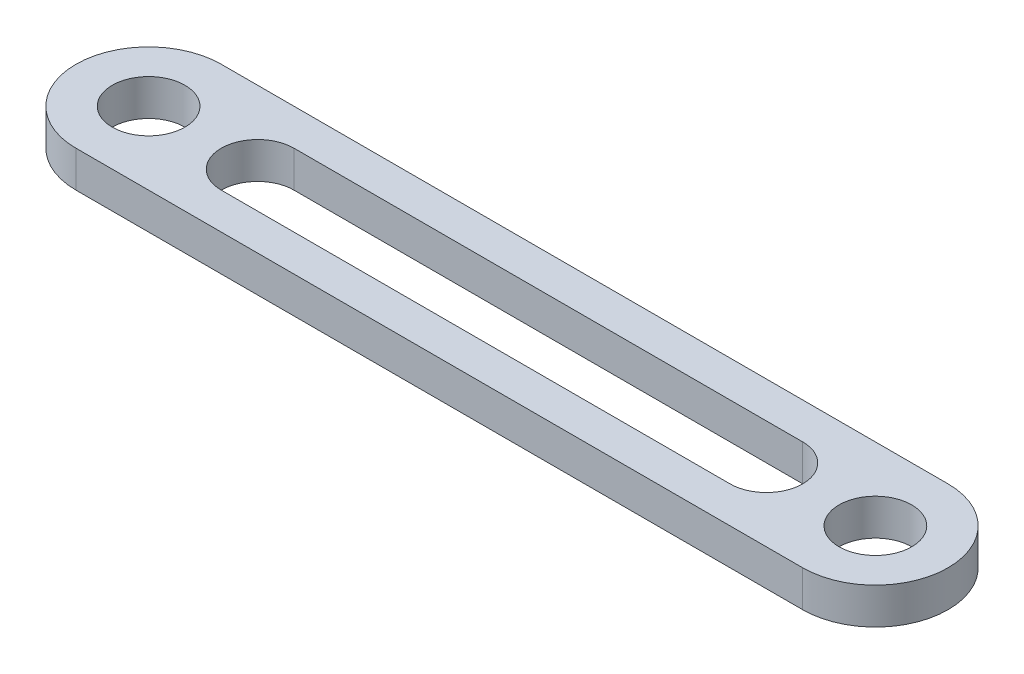
ISO-10303-21;
HEADER;
FILE_DESCRIPTION(('STEP AP214'),'2;1');
FILE_NAME('part.step','',(''),(''),'','','');
FILE_SCHEMA(('AUTOMOTIVE_DESIGN { 1 0 10303 214 1 1 1 1 }'));
ENDSEC;
DATA;
#1=APPLICATION_CONTEXT('core data for automotive mechanical design processes');
#2=APPLICATION_PROTOCOL_DEFINITION('international standard','automotive_design',2000,#1);
#3=PRODUCT_CONTEXT('',#1,'mechanical');
#4=PRODUCT('Part','Part','',(#3));
#5=PRODUCT_RELATED_PRODUCT_CATEGORY('part','',(#4));
#6=PRODUCT_DEFINITION_FORMATION('','',#4);
#7=PRODUCT_DEFINITION_CONTEXT('part definition',#1,'design');
#8=PRODUCT_DEFINITION('design','',#6,#7);
#9=PRODUCT_DEFINITION_SHAPE('','',#8);
#10=(LENGTH_UNIT() NAMED_UNIT(*) SI_UNIT(.MILLI.,.METRE.));
#11=(NAMED_UNIT(*) PLANE_ANGLE_UNIT() SI_UNIT($,.RADIAN.));
#12=(NAMED_UNIT(*) SI_UNIT($,.STERADIAN.) SOLID_ANGLE_UNIT());
#13=UNCERTAINTY_MEASURE_WITH_UNIT(LENGTH_MEASURE(1.E-05),#10,'distance_accuracy_value','');
#14=(GEOMETRIC_REPRESENTATION_CONTEXT(3) GLOBAL_UNCERTAINTY_ASSIGNED_CONTEXT((#13)) GLOBAL_UNIT_ASSIGNED_CONTEXT((#10,
#11,#12)) REPRESENTATION_CONTEXT('',''));
#15=CARTESIAN_POINT('',(0.,0.,0.));
#16=DIRECTION('',(0.,0.,1.));
#17=DIRECTION('',(1.,0.,0.));
#18=AXIS2_PLACEMENT_3D('',#15,#16,#17);
#19=CARTESIAN_POINT('',(-50.,5.,0.));
#20=DIRECTION('',(0.,1.,0.));
#21=DIRECTION('',(0.,0.,1.));
#22=AXIS2_PLACEMENT_3D('',#19,#20,#21);
#23=PLANE('',#22);
#24=CARTESIAN_POINT('',(-50.,5.,0.));
#25=DIRECTION('',(0.,1.,0.));
#26=DIRECTION('',(0.,0.,1.));
#27=AXIS2_PLACEMENT_3D('',#24,#25,#26);
#28=CIRCLE('',#27,5.);
#29=CARTESIAN_POINT('',(-50.,5.,5.));
#30=VERTEX_POINT('',#29);
#31=EDGE_CURVE('E148',#30,#30,#28,.T.);
#32=ORIENTED_EDGE('',*,*,#31,.F.);
#33=EDGE_LOOP('',(#32));
#34=FACE_BOUND('',#33,.T.);
#35=CARTESIAN_POINT('',(-50.,5.,0.));
#36=DIRECTION('',(0.,1.,0.));
#37=DIRECTION('',(0.,0.,1.));
#38=AXIS2_PLACEMENT_3D('',#35,#36,#37);
#39=CIRCLE('',#38,10.);
#40=CARTESIAN_POINT('',(-50.,5.,-10.));
#41=VERTEX_POINT('',#40);
#42=CARTESIAN_POINT('',(-50.,5.,10.));
#43=VERTEX_POINT('',#42);
#44=EDGE_CURVE('E155',#41,#43,#39,.T.);
#45=ORIENTED_EDGE('',*,*,#44,.T.);
#46=DIRECTION('',(1.,0.,0.));
#47=VECTOR('',#46,1.);
#48=CARTESIAN_POINT('',(-50.,5.,10.));
#49=LINE('',#48,#47);
#50=CARTESIAN_POINT('',(50.,5.,9.99999999999998));
#51=VERTEX_POINT('',#50);
#52=EDGE_CURVE('E154',#43,#51,#49,.T.);
#53=ORIENTED_EDGE('',*,*,#52,.T.);
#54=CARTESIAN_POINT('',(50.,5.,0.));
#55=DIRECTION('',(0.,1.,0.));
#56=DIRECTION('',(0.,0.,1.));
#57=AXIS2_PLACEMENT_3D('',#54,#55,#56);
#58=CIRCLE('',#57,10.);
#59=CARTESIAN_POINT('',(50.,5.,-10.));
#60=VERTEX_POINT('',#59);
#61=EDGE_CURVE('E158',#51,#60,#58,.T.);
#62=ORIENTED_EDGE('',*,*,#61,.T.);
#63=DIRECTION('',(-1.,0.,0.));
#64=VECTOR('',#63,1.);
#65=CARTESIAN_POINT('',(-50.,5.,-10.));
#66=LINE('',#65,#64);
#67=EDGE_CURVE('E159',#60,#41,#66,.T.);
#68=ORIENTED_EDGE('',*,*,#67,.T.);
#69=EDGE_LOOP('',(#45,#53,#62,#68));
#70=FACE_BOUND('',#69,.T.);
#71=CARTESIAN_POINT('',(50.,5.,0.));
#72=DIRECTION('',(0.,1.,0.));
#73=DIRECTION('',(0.,0.,1.));
#74=AXIS2_PLACEMENT_3D('',#71,#72,#73);
#75=CIRCLE('',#74,5.);
#76=CARTESIAN_POINT('',(50.,5.,4.99999999999998));
#77=VERTEX_POINT('',#76);
#78=EDGE_CURVE('E138',#77,#77,#75,.T.);
#79=ORIENTED_EDGE('',*,*,#78,.F.);
#80=EDGE_LOOP('',(#79));
#81=FACE_BOUND('',#80,.T.);
#82=DIRECTION('',(1.,0.,0.));
#83=VECTOR('',#82,1.);
#84=CARTESIAN_POINT('',(-35.,5.,5.00000000000001));
#85=LINE('',#84,#83);
#86=CARTESIAN_POINT('',(-35.,5.,5.00000000000001));
#87=VERTEX_POINT('',#86);
#88=CARTESIAN_POINT('',(35.,5.,5.));
#89=VERTEX_POINT('',#88);
#90=EDGE_CURVE('E115',#87,#89,#85,.T.);
#91=ORIENTED_EDGE('',*,*,#90,.F.);
#92=CARTESIAN_POINT('',(-35.,5.,0.));
#93=DIRECTION('',(0.,1.,0.));
#94=DIRECTION('',(0.,0.,1.));
#95=AXIS2_PLACEMENT_3D('',#92,#93,#94);
#96=CIRCLE('',#95,5.00000000000001);
#97=CARTESIAN_POINT('',(-35.,5.,-5.00000000000001));
#98=VERTEX_POINT('',#97);
#99=EDGE_CURVE('E102',#98,#87,#96,.T.);
#100=ORIENTED_EDGE('',*,*,#99,.F.);
#101=DIRECTION('',(-1.,0.,0.));
#102=VECTOR('',#101,1.);
#103=CARTESIAN_POINT('',(-35.,5.,-5.00000000000001));
#104=LINE('',#103,#102);
#105=CARTESIAN_POINT('',(35.,5.,-5.00000000000003));
#106=VERTEX_POINT('',#105);
#107=EDGE_CURVE('E127',#106,#98,#104,.T.);
#108=ORIENTED_EDGE('',*,*,#107,.F.);
#109=CARTESIAN_POINT('',(35.,5.,0.));
#110=DIRECTION('',(0.,1.,0.));
#111=DIRECTION('',(0.,0.,1.));
#112=AXIS2_PLACEMENT_3D('',#109,#110,#111);
#113=CIRCLE('',#112,5.00000000000001);
#114=EDGE_CURVE('E121',#89,#106,#113,.T.);
#115=ORIENTED_EDGE('',*,*,#114,.F.);
#116=EDGE_LOOP('',(#91,#100,#108,#115));
#117=FACE_BOUND('',#116,.T.);
#118=ADVANCED_FACE('F39',(#34,#70,#81,#117),#23,.T.);
#119=CARTESIAN_POINT('',(-50.,0.,0.));
#120=DIRECTION('',(0.,1.,0.));
#121=DIRECTION('',(0.,0.,1.));
#122=AXIS2_PLACEMENT_3D('',#119,#120,#121);
#123=PLANE('',#122);
#124=CARTESIAN_POINT('',(50.,0.,0.));
#125=DIRECTION('',(0.,1.,0.));
#126=DIRECTION('',(0.,0.,1.));
#127=AXIS2_PLACEMENT_3D('',#124,#125,#126);
#128=CIRCLE('',#127,5.);
#129=CARTESIAN_POINT('',(50.,0.,4.99999999999998));
#130=VERTEX_POINT('',#129);
#131=EDGE_CURVE('E118',#130,#130,#128,.T.);
#132=ORIENTED_EDGE('',*,*,#131,.T.);
#133=EDGE_LOOP('',(#132));
#134=FACE_BOUND('',#133,.T.);
#135=CARTESIAN_POINT('',(-50.,0.,0.));
#136=DIRECTION('',(0.,1.,0.));
#137=DIRECTION('',(0.,0.,1.));
#138=AXIS2_PLACEMENT_3D('',#135,#136,#137);
#139=CIRCLE('',#138,5.);
#140=CARTESIAN_POINT('',(-50.,0.,5.));
#141=VERTEX_POINT('',#140);
#142=EDGE_CURVE('E141',#141,#141,#139,.T.);
#143=ORIENTED_EDGE('',*,*,#142,.T.);
#144=EDGE_LOOP('',(#143));
#145=FACE_BOUND('',#144,.T.);
#146=CARTESIAN_POINT('',(-50.,0.,0.));
#147=DIRECTION('',(0.,1.,0.));
#148=DIRECTION('',(0.,0.,1.));
#149=AXIS2_PLACEMENT_3D('',#146,#147,#148);
#150=CIRCLE('',#149,10.);
#151=CARTESIAN_POINT('',(-50.,0.,-10.));
#152=VERTEX_POINT('',#151);
#153=CARTESIAN_POINT('',(-50.,0.,10.));
#154=VERTEX_POINT('',#153);
#155=EDGE_CURVE('E149',#152,#154,#150,.T.);
#156=ORIENTED_EDGE('',*,*,#155,.F.);
#157=DIRECTION('',(-1.,0.,0.));
#158=VECTOR('',#157,1.);
#159=CARTESIAN_POINT('',(-50.,0.,-10.));
#160=LINE('',#159,#158);
#161=CARTESIAN_POINT('',(50.,0.,-10.));
#162=VERTEX_POINT('',#161);
#163=EDGE_CURVE('E156',#162,#152,#160,.T.);
#164=ORIENTED_EDGE('',*,*,#163,.F.);
#165=CARTESIAN_POINT('',(50.,0.,0.));
#166=DIRECTION('',(0.,1.,0.));
#167=DIRECTION('',(0.,0.,1.));
#168=AXIS2_PLACEMENT_3D('',#165,#166,#167);
#169=CIRCLE('',#168,10.);
#170=CARTESIAN_POINT('',(50.,0.,9.99999999999998));
#171=VERTEX_POINT('',#170);
#172=EDGE_CURVE('E170',#171,#162,#169,.T.);
#173=ORIENTED_EDGE('',*,*,#172,.F.);
#174=DIRECTION('',(1.,0.,0.));
#175=VECTOR('',#174,1.);
#176=CARTESIAN_POINT('',(-50.,0.,10.));
#177=LINE('',#176,#175);
#178=EDGE_CURVE('E164',#154,#171,#177,.T.);
#179=ORIENTED_EDGE('',*,*,#178,.F.);
#180=EDGE_LOOP('',(#156,#164,#173,#179));
#181=FACE_BOUND('',#180,.T.);
#182=CARTESIAN_POINT('',(-35.,0.,0.));
#183=DIRECTION('',(0.,1.,0.));
#184=DIRECTION('',(0.,0.,1.));
#185=AXIS2_PLACEMENT_3D('',#182,#183,#184);
#186=CIRCLE('',#185,5.00000000000001);
#187=CARTESIAN_POINT('',(-35.,0.,-5.00000000000001));
#188=VERTEX_POINT('',#187);
#189=CARTESIAN_POINT('',(-35.,0.,5.00000000000001));
#190=VERTEX_POINT('',#189);
#191=EDGE_CURVE('E65',#188,#190,#186,.T.);
#192=ORIENTED_EDGE('',*,*,#191,.T.);
#193=DIRECTION('',(1.,0.,0.));
#194=VECTOR('',#193,1.);
#195=CARTESIAN_POINT('',(-35.,0.,5.00000000000001));
#196=LINE('',#195,#194);
#197=CARTESIAN_POINT('',(35.,0.,5.));
#198=VERTEX_POINT('',#197);
#199=EDGE_CURVE('E116',#190,#198,#196,.T.);
#200=ORIENTED_EDGE('',*,*,#199,.T.);
#201=CARTESIAN_POINT('',(35.,0.,0.));
#202=DIRECTION('',(0.,1.,0.));
#203=DIRECTION('',(0.,0.,1.));
#204=AXIS2_PLACEMENT_3D('',#201,#202,#203);
#205=CIRCLE('',#204,5.00000000000001);
#206=CARTESIAN_POINT('',(35.,0.,-5.00000000000003));
#207=VERTEX_POINT('',#206);
#208=EDGE_CURVE('E135',#198,#207,#205,.T.);
#209=ORIENTED_EDGE('',*,*,#208,.T.);
#210=DIRECTION('',(-1.,0.,0.));
#211=VECTOR('',#210,1.);
#212=CARTESIAN_POINT('',(-35.,0.,-5.00000000000001));
#213=LINE('',#212,#211);
#214=EDGE_CURVE('E114',#207,#188,#213,.T.);
#215=ORIENTED_EDGE('',*,*,#214,.T.);
#216=EDGE_LOOP('',(#192,#200,#209,#215));
#217=FACE_BOUND('',#216,.T.);
#218=ADVANCED_FACE('F183',(#134,#145,#181,#217),#123,.F.);
#219=CARTESIAN_POINT('',(-50.,5.,0.));
#220=DIRECTION('',(0.,-1.,0.));
#221=DIRECTION('',(0.,0.,-1.));
#222=AXIS2_PLACEMENT_3D('',#219,#220,#221);
#223=CYLINDRICAL_SURFACE('',#222,10.);
#224=ORIENTED_EDGE('',*,*,#155,.T.);
#225=DIRECTION('',(0.,-1.,0.));
#226=VECTOR('',#225,1.);
#227=CARTESIAN_POINT('',(-50.,5.,10.));
#228=LINE('',#227,#226);
#229=EDGE_CURVE('E11',#43,#154,#228,.T.);
#230=ORIENTED_EDGE('',*,*,#229,.F.);
#231=ORIENTED_EDGE('',*,*,#44,.F.);
#232=DIRECTION('',(0.,-1.,0.));
#233=VECTOR('',#232,1.);
#234=CARTESIAN_POINT('',(-50.,5.,-10.));
#235=LINE('',#234,#233);
#236=EDGE_CURVE('E165',#41,#152,#235,.T.);
#237=ORIENTED_EDGE('',*,*,#236,.T.);
#238=EDGE_LOOP('',(#224,#230,#231,#237));
#239=FACE_BOUND('',#238,.T.);
#240=ADVANCED_FACE('F41',(#239),#223,.T.);
#241=CARTESIAN_POINT('',(-50.,5.,10.));
#242=DIRECTION('',(0.,0.,-1.));
#243=DIRECTION('',(-1.,0.,0.));
#244=AXIS2_PLACEMENT_3D('',#241,#242,#243);
#245=PLANE('',#244);
#246=ORIENTED_EDGE('',*,*,#178,.T.);
#247=DIRECTION('',(0.,-1.,0.));
#248=VECTOR('',#247,1.);
#249=CARTESIAN_POINT('',(50.,5.,9.99999999999998));
#250=LINE('',#249,#248);
#251=EDGE_CURVE('E50',#51,#171,#250,.T.);
#252=ORIENTED_EDGE('',*,*,#251,.F.);
#253=ORIENTED_EDGE('',*,*,#52,.F.);
#254=ORIENTED_EDGE('',*,*,#229,.T.);
#255=EDGE_LOOP('',(#246,#252,#253,#254));
#256=FACE_BOUND('',#255,.T.);
#257=ADVANCED_FACE('F198',(#256),#245,.F.);
#258=CARTESIAN_POINT('',(50.,5.,0.));
#259=DIRECTION('',(0.,-1.,0.));
#260=DIRECTION('',(0.,0.,-1.));
#261=AXIS2_PLACEMENT_3D('',#258,#259,#260);
#262=CYLINDRICAL_SURFACE('',#261,10.);
#263=ORIENTED_EDGE('',*,*,#172,.T.);
#264=DIRECTION('',(0.,-1.,0.));
#265=VECTOR('',#264,1.);
#266=CARTESIAN_POINT('',(50.,5.,-10.));
#267=LINE('',#266,#265);
#268=EDGE_CURVE('E175',#60,#162,#267,.T.);
#269=ORIENTED_EDGE('',*,*,#268,.F.);
#270=ORIENTED_EDGE('',*,*,#61,.F.);
#271=ORIENTED_EDGE('',*,*,#251,.T.);
#272=EDGE_LOOP('',(#263,#269,#270,#271));
#273=FACE_BOUND('',#272,.T.);
#274=ADVANCED_FACE('F176',(#273),#262,.T.);
#275=CARTESIAN_POINT('',(-50.,5.,-10.));
#276=DIRECTION('',(0.,0.,1.));
#277=DIRECTION('',(1.,0.,0.));
#278=AXIS2_PLACEMENT_3D('',#275,#276,#277);
#279=PLANE('',#278);
#280=ORIENTED_EDGE('',*,*,#163,.T.);
#281=ORIENTED_EDGE('',*,*,#236,.F.);
#282=ORIENTED_EDGE('',*,*,#67,.F.);
#283=ORIENTED_EDGE('',*,*,#268,.T.);
#284=EDGE_LOOP('',(#280,#281,#282,#283));
#285=FACE_BOUND('',#284,.T.);
#286=ADVANCED_FACE('F186',(#285),#279,.F.);
#287=CARTESIAN_POINT('',(-50.,5.,0.));
#288=DIRECTION('',(0.,-1.,0.));
#289=DIRECTION('',(0.,0.,-1.));
#290=AXIS2_PLACEMENT_3D('',#287,#288,#289);
#291=CYLINDRICAL_SURFACE('',#290,5.);
#292=ORIENTED_EDGE('',*,*,#31,.T.);
#293=EDGE_LOOP('',(#292));
#294=FACE_BOUND('',#293,.T.);
#295=ORIENTED_EDGE('',*,*,#142,.F.);
#296=EDGE_LOOP('',(#295));
#297=FACE_BOUND('',#296,.T.);
#298=ADVANCED_FACE('F213',(#294,#297),#291,.F.);
#299=CARTESIAN_POINT('',(50.,5.,0.));
#300=DIRECTION('',(0.,-1.,0.));
#301=DIRECTION('',(0.,0.,-1.));
#302=AXIS2_PLACEMENT_3D('',#299,#300,#301);
#303=CYLINDRICAL_SURFACE('',#302,5.);
#304=ORIENTED_EDGE('',*,*,#78,.T.);
#305=EDGE_LOOP('',(#304));
#306=FACE_BOUND('',#305,.T.);
#307=ORIENTED_EDGE('',*,*,#131,.F.);
#308=EDGE_LOOP('',(#307));
#309=FACE_BOUND('',#308,.T.);
#310=ADVANCED_FACE('F219',(#306,#309),#303,.F.);
#311=CARTESIAN_POINT('',(-35.,5.,0.));
#312=DIRECTION('',(0.,-1.,0.));
#313=DIRECTION('',(0.,0.,-1.));
#314=AXIS2_PLACEMENT_3D('',#311,#312,#313);
#315=CYLINDRICAL_SURFACE('',#314,5.00000000000001);
#316=ORIENTED_EDGE('',*,*,#191,.F.);
#317=DIRECTION('',(0.,-1.,0.));
#318=VECTOR('',#317,1.);
#319=CARTESIAN_POINT('',(-35.,5.,-5.00000000000001));
#320=LINE('',#319,#318);
#321=EDGE_CURVE('E107',#98,#188,#320,.T.);
#322=ORIENTED_EDGE('',*,*,#321,.F.);
#323=ORIENTED_EDGE('',*,*,#99,.T.);
#324=DIRECTION('',(0.,-1.,0.));
#325=VECTOR('',#324,1.);
#326=CARTESIAN_POINT('',(-35.,5.,5.00000000000001));
#327=LINE('',#326,#325);
#328=EDGE_CURVE('E110',#87,#190,#327,.T.);
#329=ORIENTED_EDGE('',*,*,#328,.T.);
#330=EDGE_LOOP('',(#316,#322,#323,#329));
#331=FACE_BOUND('',#330,.T.);
#332=ADVANCED_FACE('F106',(#331),#315,.F.);
#333=CARTESIAN_POINT('',(-35.,5.,5.00000000000001));
#334=DIRECTION('',(0.,0.,-1.));
#335=DIRECTION('',(-1.,0.,0.));
#336=AXIS2_PLACEMENT_3D('',#333,#334,#335);
#337=PLANE('',#336);
#338=ORIENTED_EDGE('',*,*,#199,.F.);
#339=ORIENTED_EDGE('',*,*,#328,.F.);
#340=ORIENTED_EDGE('',*,*,#90,.T.);
#341=DIRECTION('',(0.,-1.,0.));
#342=VECTOR('',#341,1.);
#343=CARTESIAN_POINT('',(35.,5.,5.));
#344=LINE('',#343,#342);
#345=EDGE_CURVE('E122',#89,#198,#344,.T.);
#346=ORIENTED_EDGE('',*,*,#345,.T.);
#347=EDGE_LOOP('',(#338,#339,#340,#346));
#348=FACE_BOUND('',#347,.T.);
#349=ADVANCED_FACE('F117',(#348),#337,.T.);
#350=CARTESIAN_POINT('',(35.,5.,0.));
#351=DIRECTION('',(0.,-1.,0.));
#352=DIRECTION('',(0.,0.,-1.));
#353=AXIS2_PLACEMENT_3D('',#350,#351,#352);
#354=CYLINDRICAL_SURFACE('',#353,5.00000000000001);
#355=ORIENTED_EDGE('',*,*,#208,.F.);
#356=ORIENTED_EDGE('',*,*,#345,.F.);
#357=ORIENTED_EDGE('',*,*,#114,.T.);
#358=DIRECTION('',(0.,-1.,0.));
#359=VECTOR('',#358,1.);
#360=CARTESIAN_POINT('',(35.,5.,-5.00000000000003));
#361=LINE('',#360,#359);
#362=EDGE_CURVE('E53',#106,#207,#361,.T.);
#363=ORIENTED_EDGE('',*,*,#362,.T.);
#364=EDGE_LOOP('',(#355,#356,#357,#363));
#365=FACE_BOUND('',#364,.T.);
#366=ADVANCED_FACE('F240',(#365),#354,.F.);
#367=CARTESIAN_POINT('',(-35.,5.,-5.00000000000001));
#368=DIRECTION('',(0.,0.,1.));
#369=DIRECTION('',(1.,0.,0.));
#370=AXIS2_PLACEMENT_3D('',#367,#368,#369);
#371=PLANE('',#370);
#372=ORIENTED_EDGE('',*,*,#214,.F.);
#373=ORIENTED_EDGE('',*,*,#362,.F.);
#374=ORIENTED_EDGE('',*,*,#107,.T.);
#375=ORIENTED_EDGE('',*,*,#321,.T.);
#376=EDGE_LOOP('',(#372,#373,#374,#375));
#377=FACE_BOUND('',#376,.T.);
#378=ADVANCED_FACE('F238',(#377),#371,.T.);
#379=CLOSED_SHELL('',(#118,#218,#240,#257,#274,#286,#298,#310,#332,#349,#366,#378));
#380=MANIFOLD_SOLID_BREP('B2',#379);
#381=ADVANCED_BREP_SHAPE_REPRESENTATION('',(#18,#380),#14);
#382=SHAPE_DEFINITION_REPRESENTATION(#9,#381);
ENDSEC;
END-ISO-10303-21;
